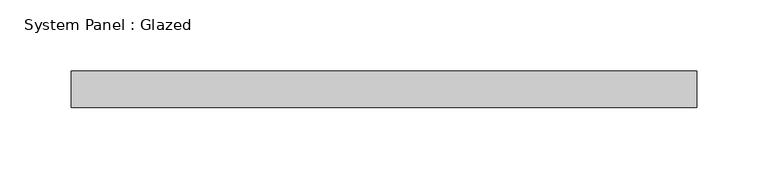
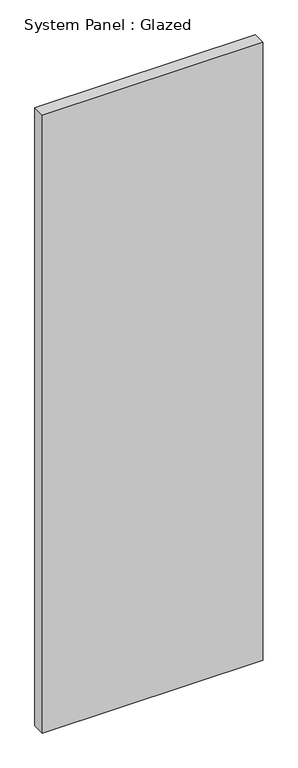
"""IFC4 building model written with IfcOpenShell, lengths in millimetres: plate geometry, System Panel : Glazed."""

from ifc_helpers import new_model, si_unit, origin, origin_with_axes, place, context, project, spatial, polyline, outline, extrude, source, transform, mapped, element, save


def system_panel_glazed_b38058b2(model_context):
    return source(origin(), model_context, "Body", "SweptSolid", [
        extrude(outline(polyline([(219.075, 19.05), (-219.075, 19.05), (-219.075, 44.45), (219.075, 44.45), (219.075, 19.05)])), origin_with_axes(), (0.0, 0.0, 1.0), 1298.0105727),
    ])


if __name__ == "__main__":
    model = new_model("IFC4")
    model_context = context("Model", 3, world=origin())
    ifc_project = project(units=[si_unit("LENGTHUNIT", "METRE", prefix="MILLI")], contexts=[model_context])
    site = spatial("IfcSite", under=ifc_project)
    building = spatial("IfcBuilding", under=site)
    placement = place(None, origin())
    system_panel_glazed_shape = system_panel_glazed_b38058b2(model_context)
    element("IfcPlate", 1, ObjectType="System Panel : Glazed", at=placement, inside=building, context=model_context, shape_type="MappedRepresentation", body=[
        mapped(system_panel_glazed_shape, transform((0.0, 0.0, 0.0), x_axis=(1.0, 0.0, 0.0), y_axis=(0.0, 1.0, 0.0), z_axis=(0.0, 0.0, 1.0))),
    ])
    save(model, "model.ifc")

# Revit data of these elements
# Type "System Panel : Glazed"
#   Construction Type Id = "GSP4R"
#   Analytic Construction = "1/8 in Pilkington single glazing"
#   Visual Light Transmittance = 0.9
#   Solar Heat Gain Coefficient = 0.86
#   Heat Transfer Coefficient (U) = 1.18115 BTU/(h·ft²·°F)
#   Define Thermal Properties by = 1
# Element 1 (IfcPlate, "System Panel : Glazed")
#   Materials on its faces: "Glass"
# Materials
#   "Glass": class "Glass", colour RGB 0 128 192, transparency 0.75, Description = "Soda Lime Glass", Cost = 0
